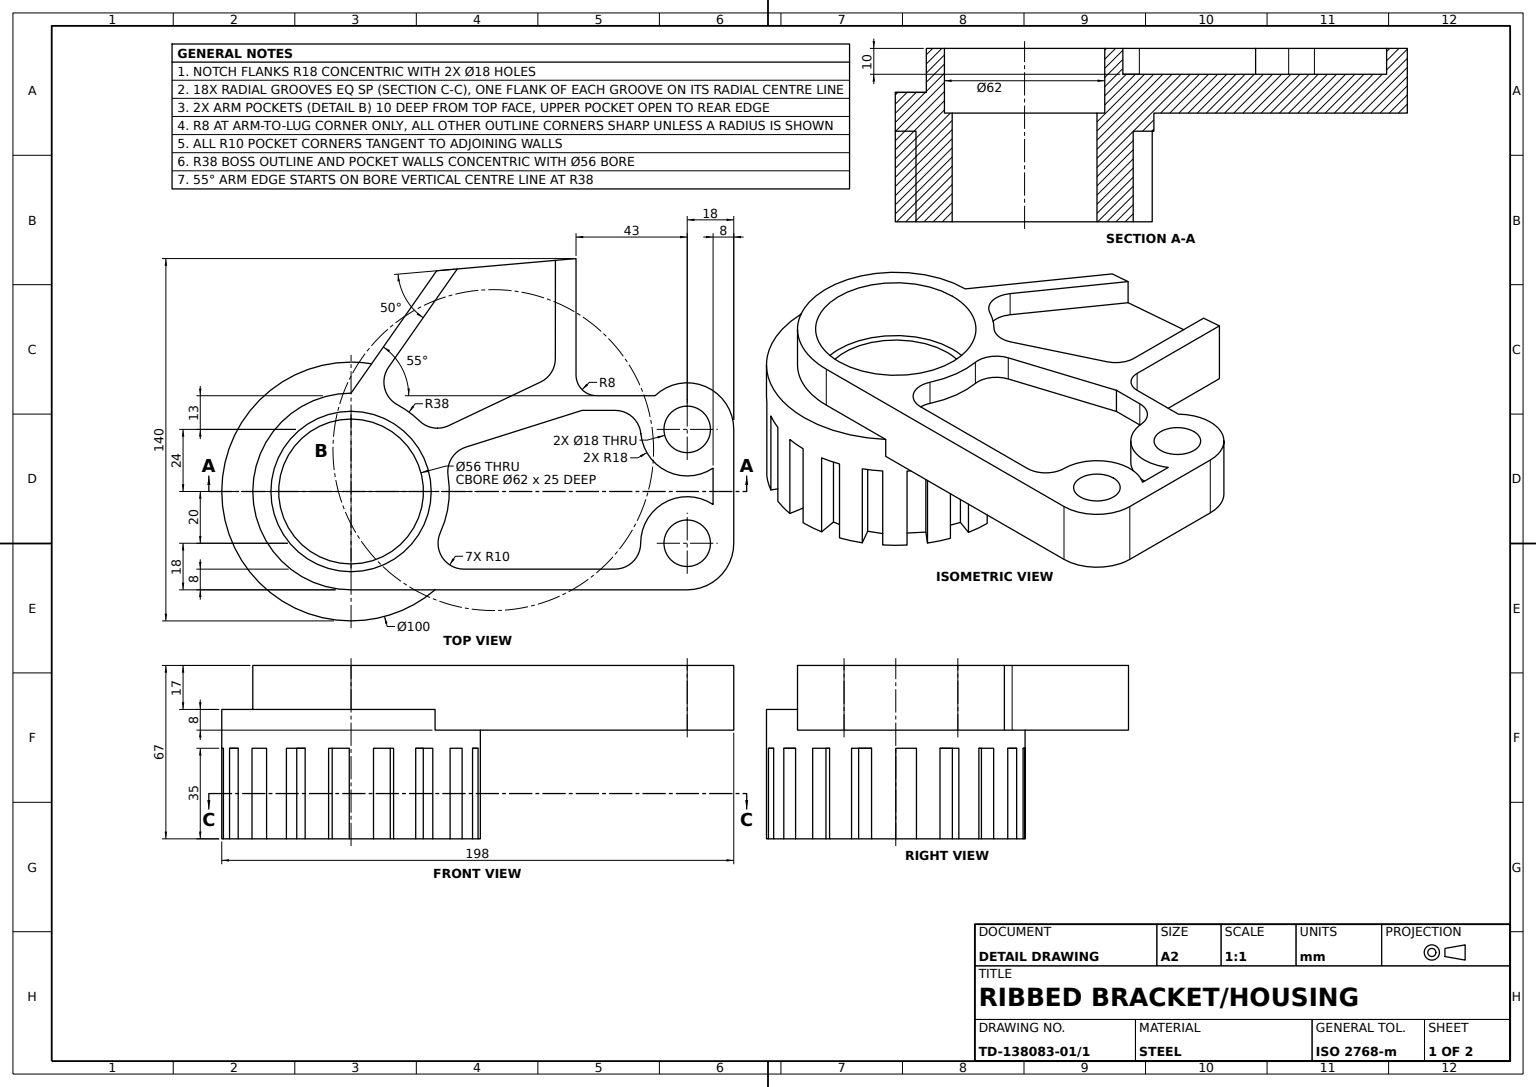
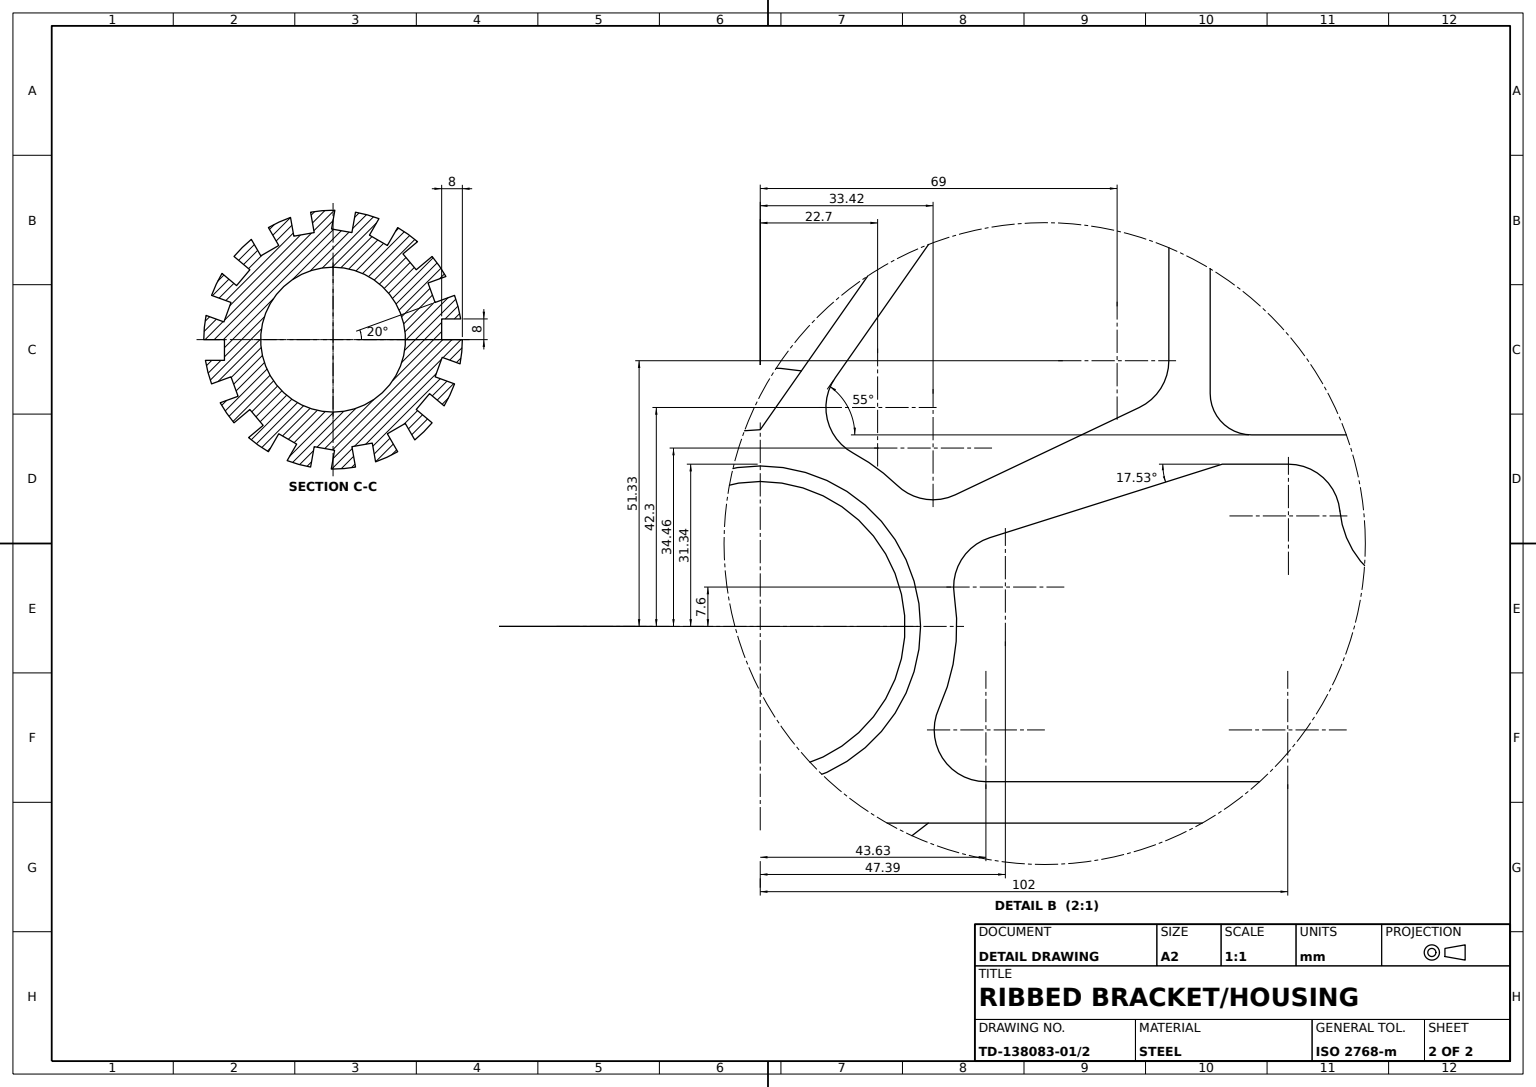
SolidWorks part; units mm, degrees
material "Plain Carbon Steel"
ref_plane "Front Plane" through (0, 0, 0) normal (0, 0, 1) x (1, 0, 0)
ref_plane "Top Plane" through (0, 0, 0) normal (0, 1, 0) x (1, 0, 0)
ref_plane "Right Plane" through (0, 0, 0) normal (1, 0, 0) x (0, 0, -1)
sketch "Hub Profile Sketch" plane through (0, 0, 0) normal (0, 1, 0) x (1, 0, 0)
  circle A0 centre (0, 0) radius 50
  dimension "D1" = 100
extrude "Hub Cylinder" add sketch "Hub Profile Sketch" along normal blind 50
ref_plane "Groove Sketch Plane" through (50, 0, 0) normal (1, 0, 0) x (0, 0, -1)
sketch "Groove Profile Sketch" plane through (50, 0, 0) normal (1, 0, 0) x (0, 0, -1)
  line L0 (0, 0) -> (0, 35)
  line L1 (-50, 0) -> (50, 0) construction
  line L2 (0, 35) -> (8, 35)
  line L3 (8, 35) -> (8, 0)
  line L4 (8, 0) -> (0, 0)
  dimension "D1" = 8
  dimension "D2" = 35
extrude "Radial Groove" cut sketch "Groove Profile Sketch" against normal blind 8
pattern_circular "Radial Groove Pattern 18x" count 18 over 360 about axis through (0, 0, 0) along (0, 1, 0) of "Radial Groove"
sketch "Bracket Arm Sketch" plane through (0, 50, 0) normal (0, 1, 0) x (1, 0, 0)
  line L0 (0, -38) -> (130, -38)
  line L1 (148, -20) -> (148, 24)
  line L2 (117.5501, 37) -> (95, 37)
  line L3 (87, 45) -> (87, 90)
  line L4 (0, 38) -> (33.1094, 85.2852)
  line L5 (87, 90) -> (33.1094, 85.2852)
  line L6 (33.1094, 85.2852) -> (41.079, 85.9824)
  line L9 (8, 38) -> (7.4866, 37.2552)
  line L10 (87, 90) -> (79.0304, 89.3028)
  circle A0 centre (0, 0) radius 38
  arc A1 (130, -38) -> (148, -20) centre (130, -20) ccw
  circle A2 centre (130, -20) radius 9
  arc A3 (148, 24) -> (117.5501, 37) centre (130, 24) ccw
  circle A4 centre (130, 24) radius 9
  arc A5 (95, 37) -> (87, 45) centre (95, 45) cw
  circle A6 centre (0, 0) radius 50 construction
  dimension "D1" = 8
  dimension "D2" = 76
  dimension "D3" = 18
  dimension "D4" = 18
  dimension "D5" = 7.4866
  dimension "D6" = 8
  dimension "D7" = 33.1094
  dimension "D8" = 41.079
  dimension "D9" = 79.0304
  dimension "D10" = 148
  dimension "D11" = 117.5501
  dimension "D12" = 24
extrude "Bracket Arm" add sketch "Bracket Arm Sketch" along normal blind 17 and the other way blind 8
sketch "Arm Pocket Sketch" plane through (0, 67, 0) normal (0, 1, 0) x (1, 0, 0)
  line L0 (33.1094, 85.2852) -> (41.079, 85.9824)
  line L1 (87, 90) -> (33.1094, 85.2852) construction
  line L2 (41.079, 85.9824) -> (7.023, 37.3454)
  line L3 (87, 90) -> (79.0304, 89.3028)
  line L4 (148, -20) -> (148, 24) construction
  line L5 (79, 45) -> (79.0304, 89.3028)
  line L7 (0, -38) -> (130, -38) construction
  line L8 (140, 2) -> (140, 9.0334)
  line L9 (140, 2) -> (140, -5.0334)
  line L11 (30.8589, 22.1749) -> (79, 45)
  line L12 (30.8589, 22.1749) -> (35.229, 14.2448)
  line L15 (89.3431, 31.3431) -> (35.229, 14.2448)
  line L16 (89.3431, 31.3431) -> (113.5659, 31.3431)
  line L17 (65, -30) -> (115.0334, -30)
  line L18 (65, -30) -> (23.3238, -30)
  circle A0 centre (0, 0) radius 38
  arc A1 (140, -5.0334) -> (115.0334, -30) centre (130, -20) ccw
  arc A2 (113.5659, 31.3431) -> (140, 9.0334) centre (130, 24) ccw
  line M13 (87, 90) -> (33.1094, 85.2852)
  dimension "D1" = 76
  dimension "D2" = 18
  dimension "D3" = 8
  dimension "D4" = 32.9666
  dimension "D5" = 34.4341
  dimension "D6" = 58.6569
  dimension "D7" = 68.9696
  dimension "D8" = 69
  dimension "D9" = 83
  dimension "D10" = 83
  dimension "D11" = 112.771
  dimension "D12" = 117.1411
  dimension "D14" = 140.977
extrude "Arm Pockets" cut sketch "Arm Pocket Sketch" against normal blind 10 contours A2 L16 L15 A0 L18 L17 A1 L9 L8 | A0 L11 L5 L2 M13
sketch "Hub Counterbore Sketch" plane through (0, 67, 0) normal (0, 1, 0) x (1, 0, 0)
  circle A0 centre (0, 0) radius 31
  dimension "D1" = 62
extrude "Hub Counterbore" cut sketch "Hub Counterbore Sketch" against normal blind 25
sketch "Hub Through Bore Sketch" plane through (0, 42, 0) normal (0, 1, 0) x (1, 0, 0)
  circle A0 centre (0, 0) radius 28
  dimension "D1" = 56
extrude "Hub Through Bore" cut sketch "Hub Through Bore Sketch" against normal blind 59
fillet "Pocket Fillet R10 A" radius 10 1 edges at (23.3238, 62, 30)
fillet "Pocket Fillet R10 B" radius 10 1 edges at (115.0334, 62, 30)
fillet "Pocket Fillet R10 C" radius 10 1 edges at (113.5659, 62, -31.3431)
fillet "Pocket Fillet R10 D" radius 10 1 edges at (35.229, 62, -14.2448)
fillet "Pocket Fillet R10 E" radius 10 1 edges at (30.8589, 62, -22.1749)
fillet "Pocket Fillet R10 F" radius 10 1 edges at (79, 62, -45)
fillet "Pocket Fillet R10 G" radius 10 1 edges at (7.023, 62, -37.3454)
